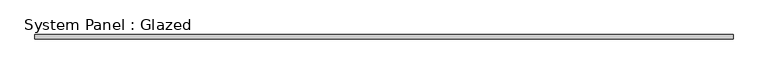
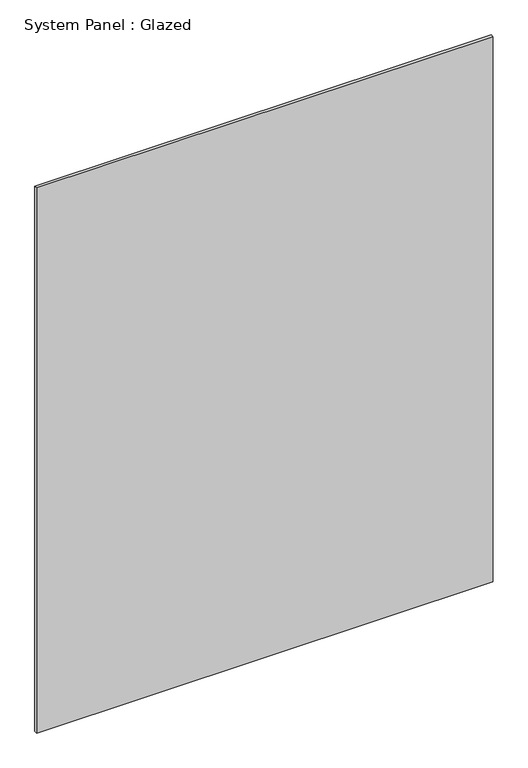
"""IFC4 building model written with IfcOpenShell, lengths in millimetres: plate geometry, System Panel : Glazed."""

from ifc_helpers import new_model, si_unit, origin, origin_with_axes, place, context, project, spatial, polyline, outline, extrude, source, transform, mapped, element, save


def system_panel_glazed_83a6671e(model_context):
    return source(origin(), model_context, "Body", "SweptSolid", [
        extrude(outline(polyline([(2001.9792392, 19.05), (-2001.9792392, 19.05), (-2001.9792392, 44.45), (2001.9792392, 44.45), (2001.9792392, 19.05)])), origin_with_axes(), (0.0, 0.0, 1.0), 5054.6),
    ])


if __name__ == "__main__":
    model = new_model("IFC4")
    model_context = context("Model", 3, world=origin())
    ifc_project = project(units=[si_unit("LENGTHUNIT", "METRE", prefix="MILLI")], contexts=[model_context])
    site = spatial("IfcSite", under=ifc_project)
    building = spatial("IfcBuilding", under=site)
    placement = place(None, origin())
    system_panel_glazed_shape = system_panel_glazed_83a6671e(model_context)
    element("IfcPlate", 1, ObjectType="System Panel : Glazed", at=placement, inside=building, context=model_context, shape_type="MappedRepresentation", body=[
        mapped(system_panel_glazed_shape, transform((0.0, 0.0, 0.0), x_axis=(1.0, 0.0, 0.0), y_axis=(0.0, 1.0, 0.0), z_axis=(0.0, 0.0, 1.0))),
    ])
    save(model, "model.ifc")

# Revit data of these elements
# Type "System Panel : Glazed"
#   Construction Type Id = "GSP4R"
#   Analytic Construction = "1/8 in Pilkington single glazing"
#   Visual Light Transmittance = 0.9
#   Solar Heat Gain Coefficient = 0.86
#   Heat Transfer Coefficient (U) = 1.18115 BTU/(h·ft²·°F)
# Element 1 (IfcPlate, "System Panel : Glazed")
#   Materials on its faces: "Glass"
# Materials
#   "Glass": class "Glass", colour RGB 0 128 192, transparency 0.75, Description = "Soda Lime Glass", Cost = 0
